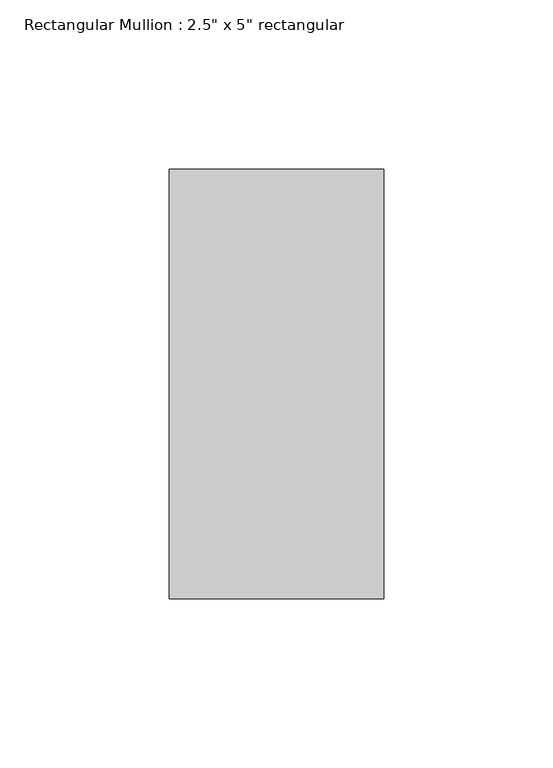
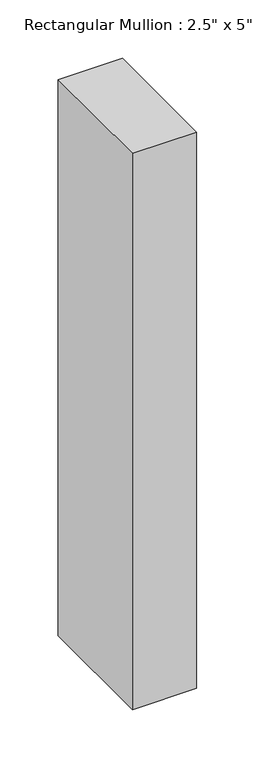
"""IFC4 building model written with IfcOpenShell, lengths in millimetres: member geometry."""

from ifc_helpers import new_model, si_unit, frame, origin, place, context, project, spatial, polyline, outline, extrude, source, transform, mapped, element, save


def member_b79e7e47(model_context):
    return source(origin(), model_context, "Body", "SweptSolid", [
        extrude(outline(polyline([(0.0, 63.5), (0.0, -63.5), (-63.5, -63.5), (-63.5, 63.5), (0.0, 63.5)])), frame((0.0, 0.0, -581.025), z_axis=(0.0, 0.0, 1.0), x_axis=(1.0, 0.0, 0.0)), (0.0, 0.0, 1.0), 581.025),
    ])


if __name__ == "__main__":
    model = new_model("IFC4")
    model_context = context("Model", 3, world=origin())
    ifc_project = project(units=[si_unit("LENGTHUNIT", "METRE", prefix="MILLI")], contexts=[model_context])
    site = spatial("IfcSite", under=ifc_project)
    building = spatial("IfcBuilding", under=site)
    placement = place(None, origin())
    member_shape = member_b79e7e47(model_context)
    element("IfcMember", 1, ObjectType="Rectangular Mullion : 2.5\" x 5\" rectangular", at=placement, inside=building, context=model_context, shape_type="MappedRepresentation", body=[
        mapped(member_shape, transform((0.0, 0.0, 0.0), x_axis=(1.0, 0.0, 0.0), y_axis=(0.0, 1.0, 0.0), z_axis=(0.0, 0.0, 1.0))),
    ])
    save(model, "model.ifc")

# Revit data of these elements
# Type "Rectangular Mullion : 2.5\" x 5\" rectangular"
#   built-in parameter 1007304 = 0.416667 (stored number, unit not read)
#   built-in parameter 1007301 = 0.104167 (stored number, unit not read)
#   built-in parameter 1007300 = 0.104167 (stored number, unit not read)
# Element 1 (IfcMember, "Rectangular Mullion : 2.5\" x 5\" rectangular")
#   Materials on its faces: "Aluminum"
# Materials
#   "Aluminum": class "Metal", colour RGB 247 247 247, transparency 0, Description = "Aluminum 6061", Cost = 0
